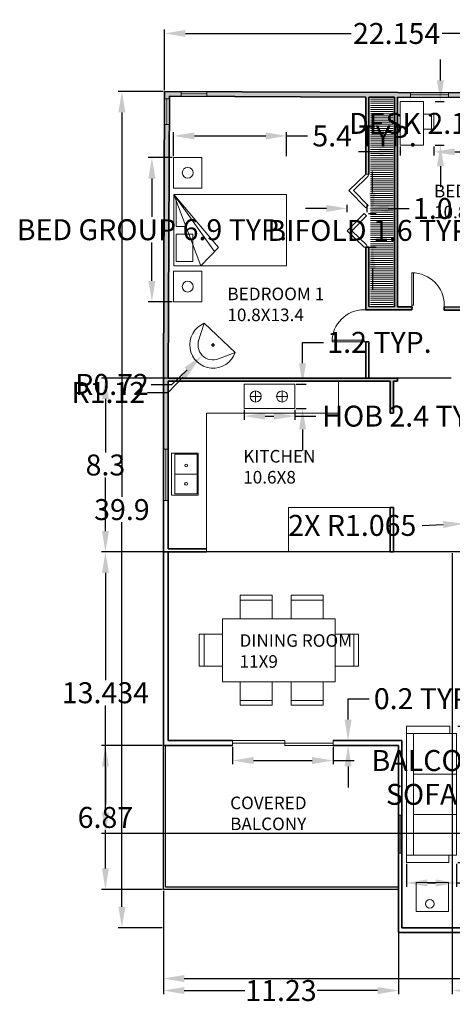
# Model space of a CAD drawing. Units: metres. Extents: x 25.1 to 96.1, y 24.3 to 71.3.
# Tile 1 of 5: x 25.1 to 45.8, y 24.3 to 71.3. Entities that reach past the tile are written whole.
import ezdxf

# ---------------------------------------------------------------- set-up
doc = ezdxf.new("R2010")
doc.units = ezdxf.units.M
doc.header["$MEASUREMENT"] = 0
for name, color, linetype, lineweight in [('A-AREA-IDEN', 1, 'Continuous', 18), ('A-EQPM', 163, 'Continuous', 18), ('A-FLOR-CASE', 8, 'Continuous', 18), ('A-FLOR-FIXT', 163, 'Continuous', 18), ('A-FLOR-RAIL', 7, 'Continuous', 25), ('A-GLAZ', 4, 'Continuous', 18), ('A-WALL', 7, 'Continuous', 35), ('A-WALL-PATT', 252, 'Continuous', 13), ('dimension', 80, 'Continuous', 18), ('door', 17, 'Continuous', 18), ('furniture', 163, 'Continuous', 18)]:
    doc.layers.add(name, color=color, linetype=linetype, lineweight=lineweight)
doc.styles.get("Standard").update_dxf_attribs({"font": 'arial.ttf'})
doc.dimstyles.get("Standard").update_dxf_attribs({"dimtxt": 1, "dimasz": 1, "dimexe": 0.18, "dimexo": 0.0625, "dimgap": 0.09, "dimtad": 0, "dimtih": 1, "dimtoh": 1, "dimdec": 1, "dimzin": 0, "dimdsep": 46, "dimtxsty": 'Standard', "dimcen": 0.09, "dimadec": 0, "dimazin": 0, "dimtfac": 1, "dimtdec": 1, "dimtofl": 0, "dimtmove": 0, "dimatfit": 3, "dimfxl": 1, "dimtolj": 1, "dimtzin": 0, "dimarcsym": 0})

# ---------------------------------------------------------------- blocks, each defined once
blk = doc.blocks.new('*D1')
at = {"layer": 'Defpoints', "color": 0, "transparency": 16777216}
for p in [(30.011, 67.873), (32.047, 67.873), (31.99, 27.968)]:
    blk.add_point(p, dxfattribs=at)
at = {"layer": 'dimension', "color": 0, "lineweight": -2, "transparency": 16777216}
for p, q in [((31.985, 67.873), (29.831, 67.873)), ((30.011, 66.873), (30.011, 48.521)), ((30.011, 28.968), (30.011, 47.319)), ((31.928, 27.968), (29.831, 27.968))]:
    blk.add_line(p, q, dxfattribs=at)
at = {"layer": 'dimension', "color": 0, "transparency": 16777216}
for points in [[(29.844, 66.873), (30.177, 66.873), (30.011, 67.873)], [(29.844, 28.968), (30.177, 28.968), (30.011, 27.968)]]:
    blk.add_solid(points, dxfattribs=at)
at = {"layer": 'dimension', "color": 0, "transparency": 16777216, "insert": (30.011, 47.92), "char_height": 1, "attachment_point": 5}
blk.add_mtext('\\A1;39.9', dxfattribs=at)
blk = doc.blocks.new('s1')
for points in [[(27.599, -10.709), (29.238, -10.709), (29.238, -10.433), (27.599, -10.433)], [(27.863, -10.709), (27.599, -10.709), (27.599, -15.302), (27.863, -15.302)], [(27.863, -10.709), (29.494, -10.709), (29.494, -12.24), (27.863, -12.24)], [(27.863, -12.24), (29.494, -12.24), (29.494, -13.771), (27.863, -13.771)], [(27.863, -13.771), (29.494, -13.771), (29.494, -15.302), (27.863, -15.302)], [(27.599, -15.577), (29.207, -15.577), (29.207, -15.302), (27.599, -15.302)]]:
    blk.add_lwpolyline(points, close=True)
blk = doc.blocks.new('ss')
blk.add_lwpolyline([(27.948, -17.463), (29.489, -17.463), (29.489, -18.849), (27.948, -18.849)], close=True)
blk.add_circle((28.593, -18.475), 0.206)
blk = doc.blocks.new('sink')
for points in [[(16.263, 3.026), (17.543, 3.026), (17.543, 1.019), (16.263, 1.019)], [(17.495, 2.968), (16.431, 2.968), (16.431, 2.028), (17.495, 2.028)], [(17.495, 2.028), (16.431, 2.028), (16.431, 1.081), (17.495, 1.081)]]:
    blk.add_lwpolyline(points, close=True)
for centre in [(16.963, 2.431), (16.961, 1.556)]:
    blk.add_circle(centre, 0.0675)
blk = doc.blocks.new('gas')
for p, q in [((20.016, 5.727), (20.544, 5.727)), ((20.28, 5.991), (20.28, 5.463)), ((21.282, 5.727), (21.81, 5.727)), ((21.546, 5.991), (21.546, 5.463))]:
    blk.add_line(p, q)
blk.add_lwpolyline([(19.729, 6.31), (22.157, 6.31), (22.157, 5.155), (19.729, 5.155)], close=True)
for centre in [(20.28, 5.727), (21.546, 5.727)]:
    blk.add_circle(centre, 0.264)
blk = doc.blocks.new('f')
at = {"layer": 'furniture'}
for p, q in [((25.769, 19.917), (26.843, 19.917)), ((25.769, 19.817), (26.843, 19.817)), ((25.769, 19.717), (26.843, 19.717)), ((25.769, 19.617), (26.843, 19.617)), ((25.769, 19.517), (26.843, 19.517)), ((25.769, 19.417), (26.843, 19.417)), ((25.769, 19.317), (26.843, 19.317)), ((25.769, 19.217), (26.843, 19.217)), ((25.769, 19.117), (26.843, 19.117)), ((25.769, 19.017), (26.843, 19.017)), ((25.769, 18.917), (26.843, 18.917)), ((25.769, 18.817), (26.843, 18.817)), ((25.769, 18.717), (26.843, 18.717)), ((25.769, 18.617), (26.843, 18.617)), ((25.769, 18.517), (26.843, 18.517)), ((25.769, 18.417), (26.843, 18.417)), ((25.769, 18.317), (26.843, 18.317)), ((25.769, 18.217), (26.843, 18.217)), ((25.769, 18.117), (26.843, 18.117)), ((25.769, 18.017), (26.843, 18.017)), ((25.769, 17.917), (26.843, 17.917)), ((25.769, 17.817), (26.843, 17.817)), ((25.769, 17.717), (26.843, 17.717)), ((25.769, 17.617), (26.843, 17.617)), ((25.769, 17.517), (26.843, 17.517)), ((25.769, 17.417), (26.843, 17.417)), ((25.769, 17.317), (26.843, 17.317)), ((25.769, 17.217), (26.843, 17.217)), ((25.769, 17.117), (26.843, 17.117)), ((25.769, 17.017), (26.843, 17.017)), ((25.769, 16.917), (26.843, 16.917)), ((25.769, 16.817), (26.843, 16.817)), ((25.769, 16.717), (26.843, 16.717)), ((25.769, 16.617), (26.843, 16.617)), ((25.769, 16.517), (26.843, 16.517)), ((25.769, 16.417), (26.843, 16.417)), ((25.769, 16.317), (26.843, 16.317)), ((25.769, 16.217), (26.843, 16.217)), ((25.769, 16.117), (26.843, 16.117)), ((25.769, 16.017), (26.843, 16.017)), ((25.769, 15.917), (26.843, 15.917)), ((25.769, 15.817), (26.843, 15.817)), ((25.769, 15.717), (26.843, 15.717)), ((25.769, 15.617), (26.843, 15.617)), ((25.769, 15.517), (26.843, 15.517)), ((25.769, 15.417), (26.843, 15.417)), ((25.769, 15.317), (26.843, 15.317)), ((25.769, 15.217), (26.843, 15.217)), ((25.769, 15.117), (26.843, 15.117)), ((25.769, 15.017), (26.843, 15.017)), ((25.769, 14.917), (26.843, 14.917)), ((25.769, 14.817), (26.843, 14.817)), ((25.769, 14.717), (26.843, 14.717)), ((25.769, 14.617), (26.843, 14.617)), ((25.769, 14.517), (26.843, 14.517)), ((25.769, 14.417), (26.843, 14.417)), ((25.769, 14.317), (26.843, 14.317)), ((25.769, 14.217), (26.843, 14.217)), ((25.769, 14.117), (26.843, 14.117)), ((25.769, 14.017), (26.843, 14.017)), ((25.769, 13.917), (26.843, 13.917)), ((25.769, 13.817), (26.843, 13.817)), ((25.769, 13.717), (26.843, 13.717)), ((25.769, 13.617), (26.843, 13.617)), ((25.769, 13.517), (26.843, 13.517)), ((25.769, 13.417), (26.843, 13.417)), ((25.769, 13.317), (26.843, 13.317)), ((25.769, 13.217), (26.843, 13.217)), ((25.769, 13.117), (26.843, 13.117)), ((25.769, 13.017), (26.843, 13.017)), ((25.769, 12.917), (26.843, 12.917)), ((25.769, 12.817), (26.843, 12.817)), ((25.769, 12.717), (26.843, 12.717)), ((25.769, 12.617), (26.843, 12.617)), ((25.769, 12.517), (26.843, 12.517)), ((25.769, 12.417), (26.843, 12.417)), ((25.769, 12.317), (26.843, 12.317)), ((25.769, 12.217), (26.843, 12.217)), ((25.769, 12.117), (26.843, 12.117)), ((25.769, 12.017), (26.843, 12.017)), ((25.769, 11.917), (26.843, 11.917)), ((25.769, 11.817), (26.843, 11.817)), ((25.769, 11.717), (26.843, 11.717)), ((25.769, 11.617), (26.843, 11.617)), ((25.769, 11.517), (26.843, 11.517)), ((25.769, 11.417), (26.843, 11.417)), ((25.769, 11.317), (26.843, 11.317)), ((25.769, 11.217), (26.843, 11.217)), ((25.769, 11.117), (26.843, 11.117)), ((25.769, 11.017), (26.843, 11.017)), ((25.769, 10.917), (26.843, 10.917)), ((25.769, 10.817), (26.843, 10.817)), ((25.769, 10.717), (26.843, 10.717)), ((25.769, 10.617), (26.843, 10.617)), ((25.769, 10.517), (26.843, 10.517)), ((25.769, 10.417), (26.843, 10.417)), ((25.769, 10.317), (26.843, 10.317)), ((25.769, 10.217), (26.843, 10.217)), ((25.769, 10.117), (26.843, 10.117))]:
    blk.add_line(p, q, dxfattribs=at)
blk = doc.blocks.new('b')
for p, q in [((16.374, 15.368), (18.513, 12.83)), ((17.666, 11.96), (16.374, 15.368)), ((16.374, 15.368), (18.324, 12.637)), ((18.513, 12.83), (17.666, 11.96))]:
    blk.add_line(p, q)
for points in [[(16.362, 17.126), (17.718, 17.126), (17.718, 15.669), (16.362, 15.669)], [(16.374, 15.368), (21.762, 15.368), (21.762, 11.96), (16.374, 11.96)], [(16.486, 12.161), (17.289, 12.161), (17.289, 13.464), (16.486, 13.464)], [(16.362, 11.698), (17.718, 11.698), (17.718, 10.242), (16.362, 10.242)]]:
    blk.add_lwpolyline(points, close=True)
blk.add_lwpolyline([(16.564, 15.144), (16.486, 15.144), (16.486, 13.84), (16.953, 13.84)])
for centre in [(17.04, 16.398), (17.04, 10.97)]:
    blk.add_circle(centre, 0.259)
blk = doc.blocks.new('cc')
for p, q in [((17.83, 9.22), (17.545, 8.337)), ((17.83, 9.22), (19.307, 7.829)), ((19.307, 7.829), (18.516, 7.517))]:
    blk.add_line(p, q)
for radius, start, end in [(1.115, 112.1788, 341.2424), (0.721, 156.2062, 291.5475)]:
    blk.add_arc((18.251, 8.188), radius, start, end)
blk = doc.blocks.new('d')
for p, q in [((25.537, 16.335), (24.732, 15.559)), ((25.644, 16.224), (24.951, 15.555)), ((25.537, 16.335), (25.687, 16.335)), ((25.644, 16.224), (25.687, 16.335)), ((24.732, 15.559), (25.537, 14.725)), ((24.951, 15.555), (25.648, 14.833)), ((25.648, 14.833), (25.537, 14.725))]:
    blk.add_line(p, q)
blk = doc.blocks.new('tt')
for points in [[(27.188, 19.803), (28.295, 19.803), (28.295, 17.712), (27.188, 17.712)], [(28.295, 19.193), (28.681, 19.193), (28.681, 18.478), (28.295, 18.478)], [(28.681, 19.193), (28.789, 19.193), (28.789, 18.478), (28.681, 18.478)]]:
    blk.add_lwpolyline(points, close=True)
blk = doc.blocks.new('*U22')
for p, q in [((0, 0), (0, -6)), ((40, 0), (40, -6))]:
    blk.add_line(p, q)
blk.add_lwpolyline([(0, 0), (0, 40), (1.75, 40), (1.75, 0)], close=True)
blk.add_arc((0, 0), 40, 0, 90)
blk = doc.blocks.new('tttt')
for points in [[(21.475, -3.758), (19.715, -3.758), (19.715, -3.49), (21.475, -3.49)], [(19.715, -4.78), (21.475, -4.78), (21.475, -3.758), (19.715, -3.758)], [(24.267, -3.758), (22.507, -3.758), (22.507, -3.49), (24.267, -3.49)], [(22.507, -4.78), (24.267, -4.78), (24.267, -3.758), (22.507, -3.758)], [(18.746, -4.78), (24.929, -4.78), (24.929, -8.239), (18.746, -8.239)], [(17.724, -5.63), (17.724, -7.389), (17.456, -7.389), (17.456, -5.63)], [(18.746, -7.389), (18.746, -5.63), (17.724, -5.63), (17.724, -7.389)], [(24.929, -7.389), (24.929, -5.63), (25.951, -5.63), (25.951, -7.389)], [(25.951, -5.63), (25.951, -7.389), (26.219, -7.389), (26.219, -5.63)], [(19.715, -8.239), (21.475, -8.239), (21.475, -9.262), (19.715, -9.262)], [(22.507, -8.239), (24.267, -8.239), (24.267, -9.262), (22.507, -9.262)], [(21.475, -9.262), (19.715, -9.262), (19.715, -9.529), (21.475, -9.529)], [(24.267, -9.262), (22.507, -9.262), (22.507, -9.529), (24.267, -9.529)]]:
    blk.add_lwpolyline(points, close=True)
blk = doc.blocks.new('*D24')
at = {"layer": 'Defpoints', "color": 0, "transparency": 16777216}
for p in [(31.99, 29.798), (83.411, 29.798), (83.411, 25.547)]:
    blk.add_point(p, dxfattribs=at)
at = {"layer": 'dimension', "color": 0, "lineweight": -2, "transparency": 16777216}
for p, q in [((31.99, 29.735), (31.99, 25.367)), ((83.411, 29.735), (83.411, 25.367)), ((32.99, 25.547), (56.314, 25.547)), ((82.411, 25.547), (59.087, 25.547))]:
    blk.add_line(p, q, dxfattribs=at)
at = {"layer": 'dimension', "color": 0, "transparency": 16777216}
for points in [[(32.99, 25.713), (32.99, 25.38), (31.99, 25.547)], [(82.411, 25.713), (82.411, 25.38), (83.411, 25.547)]]:
    blk.add_solid(points, dxfattribs=at)
at = {"layer": 'dimension', "color": 0, "transparency": 16777216, "insert": (57.7, 25.547), "char_height": 1, "attachment_point": 5}
blk.add_mtext('\\A1;51.4', dxfattribs=at)
blk = doc.blocks.new('DOOR-BALCONY-SLIDING')
for p, q in [((0, 0.23), (2.501, 0.23)), ((2.501, 0.23), (2.501, 0)), ((2.501, 0), (4.797, 0))]:
    blk.add_line(p, q)
blk.add_lwpolyline([(4.797, 0.115), (4.797, 0.115), (0, 0.115), (0, 0.115)])
blk = doc.blocks.new('*D32')
at = {"layer": 'Defpoints', "color": 0, "transparency": 16777216}
for p in [(41.726, 62.046), (41.726, 60.436), (41.967, 60.436)]:
    blk.add_point(p, dxfattribs=at)
at = {"layer": 'dimension', "color": 0, "lineweight": -2, "transparency": 16777216}
for p, q in [((41.967, 63.046), (41.967, 64.046)), ((41.788, 62.046), (42.147, 62.046)), ((41.788, 60.436), (42.147, 60.436)), ((41.967, 59.436), (41.967, 58.436))]:
    blk.add_line(p, q, dxfattribs=at)
at = {"layer": 'dimension', "color": 0, "transparency": 16777216}
for points in [[(41.801, 63.046), (42.134, 63.046), (41.967, 62.046)], [(41.801, 59.436), (42.134, 59.436), (41.967, 60.436)]]:
    blk.add_solid(points, dxfattribs=at)
at = {"layer": 'dimension', "color": 0, "transparency": 16777216, "insert": (41.967, 61.241), "char_height": 1, "attachment_point": 5}
blk.add_mtext('\\A1;BIFOLD 1.6 TYP.', dxfattribs=at)
blk = doc.blocks.new('*D33')
at = {"layer": 'Defpoints', "color": 0, "transparency": 16777216}
for p in [(40.771, 62.046), (41.726, 62.287), (41.726, 62.046)]:
    blk.add_point(p, dxfattribs=at)
at = {"layer": 'dimension', "color": 0, "lineweight": -2, "transparency": 16777216}
for p, q in [((39.771, 62.287), (38.771, 62.287)), ((40.771, 62.108), (40.771, 62.467)), ((41.726, 62.108), (41.726, 62.467)), ((42.726, 62.287), (43.726, 62.287))]:
    blk.add_line(p, q, dxfattribs=at)
at = {"layer": 'dimension', "color": 0, "transparency": 16777216}
for points in [[(39.771, 62.454), (39.771, 62.121), (40.771, 62.287)], [(42.726, 62.454), (42.726, 62.121), (41.726, 62.287)]]:
    blk.add_solid(points, dxfattribs=at)
at = {"layer": 'dimension', "color": 0, "transparency": 16777216, "insert": (46.397, 62.287), "char_height": 1, "attachment_point": 5}
blk.add_mtext('\\A1;1.0 TYP.', dxfattribs=at)
blk = doc.blocks.new('*D40')
at = {"layer": 'Defpoints', "color": 0, "transparency": 16777216}
for p in [(45.988, 37.586), (46.964, 37.586), (45.988, 31.082)]:
    blk.add_point(p, dxfattribs=at)
at = {"layer": 'dimension', "color": 0, "lineweight": -2, "transparency": 16777216}
for p, q in [((46.051, 37.586), (47.144, 37.586)), ((46.964, 36.586), (46.964, 34.941)), ((46.964, 32.082), (46.964, 33.727)), ((46.051, 31.082), (47.144, 31.082))]:
    blk.add_line(p, q, dxfattribs=at)
at = {"layer": 'dimension', "color": 0, "transparency": 16777216}
for points in [[(46.797, 36.586), (47.13, 36.586), (46.964, 37.586)], [(46.797, 32.082), (47.13, 32.082), (46.964, 31.082)]]:
    blk.add_solid(points, dxfattribs=at)
at = {"layer": 'dimension', "color": 0, "transparency": 16777216, "insert": (46.964, 34.334), "char_height": 1, "attachment_point": 5}
blk.add_mtext('\\A1;SOFA 6.5 TYP.', dxfattribs=at)
blk = doc.blocks.new('*D41')
at = {"layer": 'Defpoints', "color": 0, "transparency": 16777216}
for p in [(43.592, 31.082), (45.988, 31.082), (45.988, 30.107)]:
    blk.add_point(p, dxfattribs=at)
at = {"layer": 'dimension', "color": 0, "lineweight": -2, "transparency": 16777216}
for p, q in [((43.592, 31.02), (43.592, 29.927)), ((45.988, 31.02), (45.988, 29.927)), ((44.592, 30.107), (44.988, 30.107)), ((45.988, 30.107), (46.988, 30.107))]:
    blk.add_line(p, q, dxfattribs=at)
at = {"layer": 'dimension', "color": 0, "transparency": 16777216}
for points in [[(44.592, 30.273), (44.592, 29.94), (43.592, 30.107)], [(44.988, 30.273), (44.988, 29.94), (45.988, 30.107)]]:
    blk.add_solid(points, dxfattribs=at)
at = {"layer": 'dimension', "color": 0, "transparency": 16777216, "insert": (49.714, 30.107), "char_height": 1, "attachment_point": 5}
blk.add_mtext('\\A1;2.4 TYP.', dxfattribs=at)
blk = doc.blocks.new('*D44')
at = {"layer": 'Defpoints', "color": 0, "transparency": 16777216}
for p in [(35.843, 52.744), (38.271, 52.744), (38.271, 52.38)]:
    blk.add_point(p, dxfattribs=at)
at = {"layer": 'dimension', "color": 0, "lineweight": -2, "transparency": 16777216}
for p, q in [((35.843, 52.682), (35.843, 52.2)), ((38.271, 52.682), (38.271, 52.2)), ((36.843, 52.38), (37.271, 52.38)), ((38.271, 52.38), (39.271, 52.38))]:
    blk.add_line(p, q, dxfattribs=at)
at = {"layer": 'dimension', "color": 0, "transparency": 16777216}
for points in [[(36.843, 52.547), (36.843, 52.213), (35.843, 52.38)], [(37.271, 52.547), (37.271, 52.213), (38.271, 52.38)]]:
    blk.add_solid(points, dxfattribs=at)
at = {"layer": 'dimension', "color": 0, "transparency": 16777216, "insert": (43.67, 52.38), "char_height": 1, "attachment_point": 5}
blk.add_mtext('\\A1;HOB 2.4 TYP.', dxfattribs=at)
blk = doc.blocks.new('*D45')
at = {"layer": 'Defpoints', "color": 0, "transparency": 16777216}
for p in [(38.271, 53.899), (38.635, 53.899), (38.271, 52.744)]:
    blk.add_point(p, dxfattribs=at)
at = {"layer": 'dimension', "color": 0, "lineweight": -2, "transparency": 16777216}
for p, q in [((38.635, 54.899), (38.635, 55.899)), ((38.635, 55.899), (39.635, 55.899)), ((38.334, 53.899), (38.815, 53.899)), ((38.334, 52.744), (38.815, 52.744)), ((38.635, 51.744), (38.635, 50.744))]:
    blk.add_line(p, q, dxfattribs=at)
at = {"layer": 'dimension', "color": 0, "transparency": 16777216}
for points in [[(38.469, 54.899), (38.802, 54.899), (38.635, 53.899)], [(38.469, 51.744), (38.802, 51.744), (38.635, 52.744)]]:
    blk.add_solid(points, dxfattribs=at)
at = {"layer": 'dimension', "color": 0, "transparency": 16777216, "insert": (42.306, 55.899), "char_height": 1, "attachment_point": 5}
blk.add_mtext('\\A1;1.2 TYP.', dxfattribs=at)
blk = doc.blocks.new('*D46')
at = {"layer": 'Defpoints', "color": 0, "transparency": 16777216}
for p in [(31.444, 64.716), (32.477, 64.716), (32.477, 57.831)]:
    blk.add_point(p, dxfattribs=at)
at = {"layer": 'dimension', "color": 0, "lineweight": -2, "transparency": 16777216}
for p, q in [((32.414, 64.716), (31.264, 64.716)), ((31.444, 63.716), (31.444, 61.881)), ((31.444, 58.831), (31.444, 60.666)), ((32.414, 57.831), (31.264, 57.831))]:
    blk.add_line(p, q, dxfattribs=at)
at = {"layer": 'dimension', "color": 0, "transparency": 16777216}
for points in [[(31.277, 63.716), (31.611, 63.716), (31.444, 64.716)], [(31.277, 58.831), (31.611, 58.831), (31.444, 57.831)]]:
    blk.add_solid(points, dxfattribs=at)
at = {"layer": 'dimension', "color": 0, "transparency": 16777216, "insert": (31.444, 61.274), "char_height": 1, "attachment_point": 5}
blk.add_mtext('\\A1;BED GROUP 6.9 TYP.', dxfattribs=at)
blk = doc.blocks.new('*D47')
at = {"layer": 'Defpoints', "color": 0, "transparency": 16777216}
for p in [(37.876, 65.748), (32.477, 64.716), (37.876, 64.716)]:
    blk.add_point(p, dxfattribs=at)
at = {"layer": 'dimension', "color": 0, "lineweight": -2, "transparency": 16777216}
for p, q in [((32.477, 64.778), (32.477, 65.928)), ((37.876, 64.778), (37.876, 65.928)), ((33.477, 65.748), (36.876, 65.748)), ((37.876, 65.748), (38.876, 65.748))]:
    blk.add_line(p, q, dxfattribs=at)
at = {"layer": 'dimension', "color": 0, "transparency": 16777216}
for points in [[(33.477, 65.915), (33.477, 65.582), (32.477, 65.748)], [(36.876, 65.915), (36.876, 65.582), (37.876, 65.748)]]:
    blk.add_solid(points, dxfattribs=at)
at = {"layer": 'dimension', "color": 0, "transparency": 16777216, "insert": (41.594, 65.748), "char_height": 1, "attachment_point": 5}
blk.add_mtext('\\A1;5.4 TYP.', dxfattribs=at)
blk = doc.blocks.new('*D52')
at = {"layer": 'Defpoints', "color": 0, "transparency": 16777216}
for p in [(44.903, 67.393), (45.216, 67.393), (44.903, 65.302)]:
    blk.add_point(p, dxfattribs=at)
at = {"layer": 'dimension', "color": 0, "lineweight": -2, "transparency": 16777216}
for p, q in [((45.216, 68.393), (45.216, 69.393)), ((44.965, 67.393), (45.396, 67.393)), ((44.965, 65.302), (45.396, 65.302)), ((45.216, 64.302), (45.216, 63.302))]:
    blk.add_line(p, q, dxfattribs=at)
at = {"layer": 'dimension', "color": 0, "transparency": 16777216}
for points in [[(45.05, 68.393), (45.383, 68.393), (45.216, 67.393)], [(45.05, 64.302), (45.383, 64.302), (45.216, 65.302)]]:
    blk.add_solid(points, dxfattribs=at)
at = {"layer": 'dimension', "color": 0, "transparency": 16777216, "insert": (45.216, 66.348), "char_height": 1, "attachment_point": 5}
blk.add_mtext('\\A1;DESK 2.1 TYP.', dxfattribs=at)
blk = doc.blocks.new('*D53')
at = {"layer": 'Defpoints', "color": 0, "transparency": 16777216}
for p in [(43.302, 65.302), (44.903, 65.302), (44.903, 64.989)]:
    blk.add_point(p, dxfattribs=at)
at = {"layer": 'dimension', "color": 0, "lineweight": -2, "transparency": 16777216}
for p, q in [((42.302, 64.989), (41.302, 64.989)), ((43.302, 65.24), (43.302, 64.809)), ((44.903, 65.24), (44.903, 64.809)), ((45.903, 64.989), (46.903, 64.989))]:
    blk.add_line(p, q, dxfattribs=at)
at = {"layer": 'dimension', "color": 0, "transparency": 16777216}
for points in [[(42.302, 65.155), (42.302, 64.822), (43.302, 64.989)], [(45.903, 65.155), (45.903, 64.822), (44.903, 64.989)]]:
    blk.add_solid(points, dxfattribs=at)
at = {"layer": 'dimension', "color": 0, "transparency": 16777216, "insert": (49.574, 64.989), "char_height": 1, "attachment_point": 5}
blk.add_mtext('\\A1;1.6 TYP.', dxfattribs=at)
blk = doc.blocks.new('*D76')
at = {"layer": 'Defpoints', "color": 0, "transparency": 16777216}
for p in [(35.294, 36.668), (40.091, 36.668), (40.091, 35.948)]:
    blk.add_point(p, dxfattribs=at)
at = {"layer": 'dimension', "color": 0, "lineweight": -2, "transparency": 16777216}
for p, q in [((35.294, 36.605), (35.294, 35.768)), ((40.091, 36.605), (40.091, 35.768)), ((36.294, 35.948), (39.091, 35.948)), ((40.091, 35.948), (41.091, 35.948))]:
    blk.add_line(p, q, dxfattribs=at)
at = {"layer": 'dimension', "color": 0, "transparency": 16777216}
for points in [[(36.294, 36.115), (36.294, 35.781), (35.294, 35.948)], [(39.091, 36.115), (39.091, 35.781), (40.091, 35.948)]]:
    blk.add_solid(points, dxfattribs=at)
at = {"layer": 'dimension', "color": 0, "transparency": 16777216, "insert": (50.036, 35.948), "char_height": 1, "attachment_point": 5}
blk.add_mtext('\\A1;BALCONY SLIDER 4.8 TYP.', dxfattribs=at)
blk = doc.blocks.new('*D77')
at = {"layer": 'Defpoints', "color": 0, "transparency": 16777216}
for p in [(40.091, 36.898), (40.091, 36.668), (40.81, 36.898)]:
    blk.add_point(p, dxfattribs=at)
at = {"layer": 'dimension', "color": 0, "lineweight": -2, "transparency": 16777216}
for p, q in [((40.81, 37.898), (40.81, 38.898)), ((40.81, 38.898), (41.81, 38.898)), ((40.153, 36.898), (40.99, 36.898)), ((40.153, 36.668), (40.99, 36.668)), ((40.81, 35.668), (40.81, 34.668))]:
    blk.add_line(p, q, dxfattribs=at)
at = {"layer": 'dimension', "color": 0, "transparency": 16777216}
for points in [[(40.643, 37.898), (40.977, 37.898), (40.81, 36.898)], [(40.643, 35.668), (40.977, 35.668), (40.81, 36.668)]]:
    blk.add_solid(points, dxfattribs=at)
at = {"layer": 'dimension', "color": 0, "transparency": 16777216, "insert": (44.528, 38.898), "char_height": 1, "attachment_point": 5}
blk.add_mtext('\\A1;0.2 TYP.', dxfattribs=at)
blk = doc.blocks.new('*D78')
at = {"layer": 'Defpoints', "color": 0, "transparency": 16777216}
for p in [(45.784, 45.898), (51.084, 45.898), (51.084, 24.973)]:
    blk.add_point(p, dxfattribs=at)
at = {"layer": 'dimension', "color": 0, "lineweight": -2, "transparency": 16777216}
for p, q in [((45.784, 45.835), (45.784, 24.793)), ((51.084, 45.835), (51.084, 24.793)), ((46.784, 24.973), (47.434, 24.973)), ((50.084, 24.973), (49.434, 24.973))]:
    blk.add_line(p, q, dxfattribs=at)
at = {"layer": 'dimension', "color": 0, "transparency": 16777216}
for points in [[(46.784, 25.139), (46.784, 24.806), (45.784, 24.973)], [(50.084, 25.139), (50.084, 24.806), (51.084, 24.973)]]:
    blk.add_solid(points, dxfattribs=at)
at = {"layer": 'dimension', "color": 0, "transparency": 16777216, "insert": (48.434, 24.973), "char_height": 1, "attachment_point": 5}
blk.add_mtext('\\A1;5.3', dxfattribs=at)
blk = doc.blocks.new('*D80')
at = {"layer": 'Defpoints', "color": 0, "transparency": 16777216}
for p in [(29.225, 54.198), (45.784, 54.198), (45.784, 45.898)]:
    blk.add_point(p, dxfattribs=at)
at = {"layer": 'dimension', "color": 0, "lineweight": -2, "transparency": 16777216}
for p, q in [((45.722, 54.198), (29.045, 54.198)), ((29.225, 53.198), (29.225, 50.648)), ((29.225, 46.898), (29.225, 49.447)), ((45.722, 45.898), (29.045, 45.898))]:
    blk.add_line(p, q, dxfattribs=at)
at = {"layer": 'dimension', "color": 0, "transparency": 16777216}
for points in [[(29.059, 53.198), (29.392, 53.198), (29.225, 54.198)], [(29.059, 46.898), (29.392, 46.898), (29.225, 45.898)]]:
    blk.add_solid(points, dxfattribs=at)
at = {"layer": 'dimension', "color": 0, "transparency": 16777216, "insert": (29.225, 50.048), "char_height": 1, "attachment_point": 5}
blk.add_mtext('\\A1;8.3', dxfattribs=at)
blk = doc.blocks.new('*D81')
at = {"layer": 'Defpoints', "color": 0, "transparency": 16777216}
for p in [(54.201, 70.638), (32.047, 67.873), (54.201, 67.782)]:
    blk.add_point(p, dxfattribs=at)
at = {"layer": 'dimension', "color": 0, "lineweight": -2, "transparency": 16777216}
for p, q in [((32.047, 67.935), (32.047, 70.818)), ((33.047, 70.638), (40.952, 70.638)), ((53.201, 70.638), (45.296, 70.638)), ((54.201, 67.844), (54.201, 70.818))]:
    blk.add_line(p, q, dxfattribs=at)
at = {"layer": 'dimension', "color": 0, "transparency": 16777216}
for points in [[(33.047, 70.804), (33.047, 70.471), (32.047, 70.638)], [(53.201, 70.804), (53.201, 70.471), (54.201, 70.638)]]:
    blk.add_solid(points, dxfattribs=at)
at = {"layer": 'dimension', "color": 0, "transparency": 16777216, "insert": (43.124, 70.638), "char_height": 1, "attachment_point": 5}
blk.add_mtext('\\A1;22.154', dxfattribs=at)
blk = doc.blocks.new('*D82')
at = {"layer": 'Defpoints', "color": 0, "transparency": 16777216}
for p in [(31.99, 29.798), (43.22, 29.798), (43.22, 24.973)]:
    blk.add_point(p, dxfattribs=at)
at = {"layer": 'dimension', "color": 0, "lineweight": -2, "transparency": 16777216}
for p, q in [((31.99, 29.735), (31.99, 24.793)), ((43.22, 29.735), (43.22, 24.793)), ((32.99, 24.973), (35.875, 24.973)), ((42.22, 24.973), (39.335, 24.973))]:
    blk.add_line(p, q, dxfattribs=at)
at = {"layer": 'dimension', "color": 0, "transparency": 16777216}
for points in [[(32.99, 25.139), (32.99, 24.806), (31.99, 24.973)], [(42.22, 25.139), (42.22, 24.806), (43.22, 24.973)]]:
    blk.add_solid(points, dxfattribs=at)
at = {"layer": 'dimension', "color": 0, "transparency": 16777216, "insert": (37.605, 24.973), "char_height": 1, "attachment_point": 5}
blk.add_mtext('\\A1;11.23', dxfattribs=at)
blk = doc.blocks.new('*D83')
at = {"layer": 'Defpoints', "color": 0, "transparency": 16777216}
for p in [(29.225, 36.668), (31.99, 36.668), (31.99, 29.798)]:
    blk.add_point(p, dxfattribs=at)
at = {"layer": 'dimension', "color": 0, "lineweight": -2, "transparency": 16777216}
for p, q in [((31.928, 36.668), (29.045, 36.668)), ((29.225, 35.668), (29.225, 33.833)), ((29.225, 30.798), (29.225, 32.632)), ((31.928, 29.798), (29.045, 29.798))]:
    blk.add_line(p, q, dxfattribs=at)
at = {"layer": 'dimension', "color": 0, "transparency": 16777216}
for points in [[(29.059, 35.668), (29.392, 35.668), (29.225, 36.668)], [(29.059, 30.798), (29.392, 30.798), (29.225, 29.798)]]:
    blk.add_solid(points, dxfattribs=at)
at = {"layer": 'dimension', "color": 0, "transparency": 16777216, "insert": (29.225, 33.233), "char_height": 1, "attachment_point": 5}
blk.add_mtext('\\A1;6.87', dxfattribs=at)
blk = doc.blocks.new('*D84')
at = {"layer": 'Defpoints', "color": 0, "transparency": 16777216}
for p in [(29.225, 45.898), (61.201, 45.898), (61.201, 32.464)]:
    blk.add_point(p, dxfattribs=at)
at = {"layer": 'dimension', "color": 0, "lineweight": -2, "transparency": 16777216}
for p, q in [((61.138, 45.898), (29.045, 45.898)), ((29.225, 44.898), (29.225, 39.781)), ((29.225, 33.464), (29.225, 38.58)), ((61.138, 32.464), (29.045, 32.464))]:
    blk.add_line(p, q, dxfattribs=at)
at = {"layer": 'dimension', "color": 0, "transparency": 16777216}
for points in [[(29.059, 44.898), (29.392, 44.898), (29.225, 45.898)], [(29.059, 33.464), (29.392, 33.464), (29.225, 32.464)]]:
    blk.add_solid(points, dxfattribs=at)
at = {"layer": 'dimension', "color": 0, "transparency": 16777216, "insert": (29.225, 39.181), "char_height": 1, "attachment_point": 5}
blk.add_mtext('\\A1;13.434', dxfattribs=at)
blk = doc.blocks.new('*D88')
at = {"layer": 'Defpoints', "color": 0, "transparency": 16777216}
for p in [(46.349, 47.247), (47.413, 47.29)]:
    blk.add_point(p, dxfattribs=at)
at = {"layer": 'dimension', "color": 0, "lineweight": -2, "transparency": 16777216}
for p, q in [((44.351, 47.166), (45.35, 47.207)), ((47.323, 47.29), (47.503, 47.29)), ((47.413, 47.2), (47.413, 47.38))]:
    blk.add_line(p, q, dxfattribs=at)
at = {"layer": 'dimension', "color": 0, "transparency": 16777216}
blk.add_solid([(45.344, 47.373), (45.357, 47.04), (46.349, 47.247)], dxfattribs=at)
at = {"layer": 'dimension', "color": 0, "transparency": 16777216, "insert": (41.009, 47.166), "char_height": 1, "attachment_point": 5}
blk.add_mtext('\\A1;2X R1.065', dxfattribs=at)
blk = doc.blocks.new('*D89')
at = {"layer": 'Defpoints', "color": 0, "transparency": 16777216}
for p in [(34.365, 55.778), (33.6, 54.966)]:
    blk.add_point(p, dxfattribs=at)
at = {"layer": 'dimension', "color": 0, "lineweight": -2, "transparency": 16777216}
for p, q in [((34.275, 55.778), (34.455, 55.778)), ((34.365, 55.688), (34.365, 55.868)), ((32.228, 53.51), (32.914, 54.238)), ((31.228, 53.51), (32.228, 53.51))]:
    blk.add_line(p, q, dxfattribs=at)
at = {"layer": 'dimension', "color": 0, "transparency": 16777216}
blk.add_solid([(32.793, 54.352), (33.036, 54.124), (33.6, 54.966)], dxfattribs=at)
at = {"layer": 'dimension', "color": 0, "transparency": 16777216, "insert": (29.366, 53.51), "char_height": 1, "attachment_point": 5}
blk.add_mtext('\\A1;R1.12', dxfattribs=at)
blk = doc.blocks.new('*D90')
at = {"layer": 'Defpoints', "color": 0, "transparency": 16777216}
for p in [(34.365, 55.778), (33.845, 55.278)]:
    blk.add_point(p, dxfattribs=at)
at = {"layer": 'dimension', "color": 0, "lineweight": -2, "transparency": 16777216}
for p, q in [((34.275, 55.778), (34.455, 55.778)), ((34.365, 55.688), (34.365, 55.868)), ((32.403, 53.892), (33.124, 54.585)), ((31.403, 53.892), (32.403, 53.892))]:
    blk.add_line(p, q, dxfattribs=at)
at = {"layer": 'dimension', "color": 0, "transparency": 16777216}
blk.add_solid([(33.008, 54.705), (33.239, 54.465), (33.845, 55.278)], dxfattribs=at)
at = {"layer": 'dimension', "color": 0, "transparency": 16777216, "insert": (29.541, 53.892), "char_height": 1, "attachment_point": 5}
blk.add_mtext('\\A1;R0.72', dxfattribs=at)

msp = doc.modelspace()

# ---------------------------------------------------------------- hatches: boundary and pattern name
at = {"layer": 'A-WALL-PATT'}
h = msp.add_hatch(color=256, dxfattribs=at)
h.dxf.hatch_style = 1
h.paths.add_polyline_path([(32.2705, 66.2918), (32.0405, 66.2928), (31.9902, 54.0475), (31.9902, 50.7969), (32.2202, 50.7969), (32.2202, 54.0475), (42.8202, 54.0475), (42.8202, 52.5275), (42.9702, 52.5275), (42.9702, 54.0475), (43.1708, 54.0475), (43.1708, 54.1975), (32.2208, 54.1975)])
h.paths.add_polyline_path([(32.8404, 67.8694), (32.047, 67.8727), (32.0456, 67.5128), (32.2756, 67.5118), (32.2761, 67.6417), (32.8395, 67.6394)])
h.paths.add_polyline_path([(43.7857, 67.8244), (34.0604, 67.8644), (34.0595, 67.6344), (41.6508, 67.6032), (41.6508, 63.9251), (41.8008, 63.9251), (41.8008, 67.6026), (43.0208, 67.5975), (43.0208, 57.5975), (41.8008, 57.6025), (41.8008, 60.436), (41.6508, 60.436), (41.6508, 57.4531), (43.8592, 57.444), (43.8592, 57.594), (43.1708, 57.5968), (43.1708, 67.5969), (43.7848, 67.5944)])
h.paths.add_polyline_path([(56.5108, 67.7816), (54.2008, 67.7816), (45.5957, 67.8169), (45.5947, 67.5869), (53.9708, 67.5525), (53.9708, 58.9224), (52.4515, 58.9287), (52.4508, 58.779), (52.4512, 58.7787), (53.9708, 58.7724), (53.9708, 57.5524), (49.0027, 57.5728), (49.0077, 58.7928), (50.2244, 58.7878), (50.2244, 58.9378), (48.8584, 58.9435), (48.8577, 58.7935), (48.8527, 57.5735), (45.4006, 57.5877), (45.4006, 57.4377), (53.9634, 57.4024), (54.2008, 57.4024), (54.2008, 67.5516), (56.5108, 67.5516)])
h.paths.add_polyline_path([(68.3657, 67.7816), (58.8908, 67.7816), (58.8908, 67.5516), (61.2008, 67.5516), (61.2008, 57.4016), (61.4308, 57.4016), (67.4455, 57.4016), (67.4455, 58.9016), (66.0112, 58.9016), (66.0112, 58.7516), (67.2955, 58.7516), (67.2955, 57.5516), (61.4308, 57.5516), (61.4308, 58.7516), (63.7844, 58.7516), (63.7844, 58.9016), (61.4308, 58.9016), (61.4308, 67.5516), (68.3657, 67.5516)])

# ---------------------------------------------------------------- linework, layer by layer
at = {"layer": 'A-FLOR-CASE'}
for p, q in [((40.3575, 52.5275), (40.3575, 54.0475)), ((34.0502, 45.8975), (34.0502, 52.5275)), ((40.3575, 52.5275), (34.0502, 52.5275))]:
    msp.add_line(p, q, dxfattribs=at)
msp.add_lwpolyline([(42.8202, 45.8975), (42.8202, 48.0275), (37.9709, 48.0275), (37.9709, 45.8975), (42.8202, 45.8975)], dxfattribs=at)
at = {"layer": 'A-FLOR-RAIL'}
for p, q in [((31.9902, 29.7975), (31.9902, 36.6675)), ((32.0902, 29.8975), (32.0902, 36.6675)), ((43.2202, 29.7975), (31.9902, 29.7975)), ((43.2202, 29.8975), (32.0902, 29.8975))]:
    msp.add_line(p, q, dxfattribs=at)
at = {"layer": 'A-GLAZ'}
for p, q in [((32.8395, 67.6394), (32.8404, 67.8694)), ((34.0599, 67.7494), (32.8399, 67.7544)), ((34.0595, 67.6344), (34.0604, 67.8644)), ((43.7848, 67.5944), (43.7857, 67.8244)), ((43.7852, 67.7094), (45.5952, 67.7019)), ((45.5947, 67.5869), (45.5957, 67.8169)), ((32.2756, 67.5118), (32.0456, 67.5128)), ((32.1555, 66.2923), (32.1606, 67.5123)), ((32.2705, 66.2918), (32.0405, 66.2928)), ((32.2202, 50.7969), (31.9902, 50.7969)), ((32.1052, 50.7969), (32.1052, 48.3569)), ((32.2202, 48.3569), (31.9902, 48.3569)), ((43.3702, 33.3425), (43.2202, 33.3425)), ((43.2952, 31.5225), (43.2952, 33.3425)), ((43.3702, 31.5225), (43.2202, 31.5225))]:
    msp.add_line(p, q, dxfattribs=at)
at = {"layer": 'A-WALL'}
for p, q in [((31.9902, 54.0475), (32.047, 67.8727)), ((32.047, 67.8727), (54.2008, 67.7816)), ((32.2208, 54.1975), (32.2761, 67.6417)), ((32.2761, 67.6417), (41.6508, 67.6032)), ((41.6508, 67.6032), (41.6508, 63.9251)), ((41.8008, 67.6026), (41.8008, 63.9251)), ((41.8008, 67.6026), (43.0208, 67.5975)), ((43.0208, 67.5975), (43.0208, 57.5975)), ((43.1708, 67.5969), (43.1708, 57.5968)), ((43.1708, 67.5969), (53.9708, 67.5525)), ((41.6508, 60.6092), (41.6508, 60.6092)), ((41.6508, 60.436), (41.8008, 60.436)), ((41.6508, 60.436), (41.6508, 57.4531)), ((41.8008, 60.436), (41.8008, 57.6025)), ((41.6508, 57.4531), (43.8592, 57.444)), ((41.8008, 57.6025), (43.0208, 57.5975)), ((43.1708, 57.5968), (43.8598, 57.594)), ((43.8598, 57.594), (43.8592, 57.444)), ((45.3998, 57.5877), (45.3992, 57.4377)), ((45.3992, 57.4377), (53.9708, 57.4024)), ((45.3998, 57.5877), (48.8527, 57.5735)), ((41.6508, 55.93), (41.6508, 54.1975)), ((41.8008, 55.93), (41.6508, 55.93)), ((41.8008, 55.93), (41.8008, 54.1975)), ((31.9902, 36.6675), (31.9902, 54.0475)), ((32.2202, 46.0475), (32.2202, 54.0475)), ((42.8202, 54.0475), (32.2202, 54.0475)), ((43.1708, 54.1975), (32.2208, 54.1975)), ((42.8202, 52.5275), (42.8202, 54.0475)), ((43.1708, 54.0475), (42.9702, 54.0475)), ((42.9702, 52.5275), (42.9702, 54.0475)), ((43.1708, 54.1975), (43.1708, 54.0475)), ((42.8202, 52.5275), (42.9702, 52.5275)), ((42.8202, 45.8975), (42.8202, 48.0275)), ((42.9702, 48.0275), (42.8202, 48.0275)), ((42.9702, 45.8975), (42.9702, 48.0275)), ((34.0502, 46.0475), (32.2202, 46.0475)), ((34.0502, 45.8975), (31.9902, 45.8975)), ((32.2202, 36.8975), (32.2202, 45.8975)), ((42.9702, 45.8975), (42.8202, 45.8975)), ((35.2938, 36.6675), (31.9902, 36.6675)), ((35.2938, 36.8975), (32.2202, 36.8975)), ((43.3702, 36.8975), (40.0906, 36.8975)), ((43.2202, 36.6675), (40.0906, 36.6675)), ((43.2202, 29.8975), (43.2202, 36.6675)), ((43.3702, 27.9675), (43.3702, 36.8975)), ((43.2202, 27.7375), (43.2202, 29.8975)), ((54.2008, 27.7375), (43.2202, 27.7375)), ((53.9708, 27.9675), (43.3702, 27.9675))]:
    msp.add_line(p, q, dxfattribs=at)
at = {"layer": 'door'}
for p, q in [((35.2938, 36.6675), (35.2938, 36.8975)), ((40.0906, 36.6675), (40.0906, 36.8975))]:
    msp.add_line(p, q, dxfattribs=at)

# ---------------------------------------------------------------- block references
at = {"layer": 'A-EQPM'}
msp.add_blockref('gas', (16.1141, 47.5898), dxfattribs=at)
at = {"layer": 'A-FLOR-CASE'}
msp.add_blockref('f', (16.1141, 47.5898), dxfattribs=at)
msp.add_blockref('f', (16.1141, 47.5898), dxfattribs=at)
at = {"layer": 'A-FLOR-FIXT'}
msp.add_blockref('sink', (16.1141, 47.5898), dxfattribs=at)
at = {"layer": 'door'}
for name, p in [('d', (16.1141, 47.5898)), ('DOOR-BALCONY-SLIDING', (35.294, 36.668))]:
    msp.add_blockref(name, p, dxfattribs=at)
at = {"layer": 'door', "xscale": -1, "rotation": 180}
msp.add_blockref('d', (16.0391, 76.7713), dxfattribs=at)
at = {"layer": 'door', "xscale": 0.0385366420547583, "yscale": 0.0385366420547583, "zscale": 0.0385366420547583}
msp.add_blockref('*U22', (43.8592, 57.6752), dxfattribs=at)
at = {"layer": 'door', "xscale": 0.0381340016713186, "yscale": 0.0381340016713186, "zscale": 0.0381340016713186, "rotation": 90}
msp.add_blockref('*U22', (41.572, 55.93), dxfattribs=at)
at = {"layer": 'furniture'}
for name in ['tt', 'b', 'cc', 'ss']:
    msp.add_blockref(name, (16.1141, 47.5898), dxfattribs=at)
for name, p, xscale, yscale, zscale in [('tttt', (18.5321, 46.8655), 0.8688370319284477, 0.8688370319284477, 0.8688370319284477), ('s1', (8.6961, 50.7774), 1.264373167528455, 1.264373167528455, 1.264373167528455)]:
    msp.add_blockref(name, p, dxfattribs=dict(at, xscale=xscale, yscale=yscale, zscale=zscale))

# ---------------------------------------------------------------- texts
at = {"layer": 'A-AREA-IDEN', "char_height": 0.6, "attachment_point": 1}
for s, width, insert in [('BEDROOM 2\\P10.8X10', 5.007262, (44.9092, 63.415)), ('BEDROOM 1\\P10.8X13.4', 5.007262, (35.0481, 58.511)), ('KITCHEN\\P10.6X8', 5.007262, (35.802, 50.7644)), ('DINING ROOM\\P11X9', 11.597488, (35.628, 41.9738)), ('COVERED\\PBALCONY', 5.007262, (35.1792, 34.2251))]:
    msp.add_mtext_dynamic_manual_height_columns(s, width=width, gutter_width=1, heights=[0], dxfattribs=dict(at, insert=insert))

# ---------------------------------------------------------------- dimensions: what is measured, and where the dimension line sits
at = {"layer": 'dimension'}
for base, p1, p2, override, picture, middle in [((54.2008, 70.6377), (32.047, 67.8727), (54.2008, 67.7816), {"dimdec": 3, "dimlfac": 1, "dimrnd": 0, "dimzin": 0, "dimdsep": 46, "dimlunit": 2}, '*D81', (43.1239, 70.6377)), ((51.0841, 24.9725), (45.7841, 45.8975), (51.0841, 45.8975), {"dimdec": 1, "dimlfac": 1, "dimrnd": 0, "dimzin": 0, "dimdsep": 46, "dimlunit": 2}, '*D78', (48.4341, 24.9725)), ((83.4108, 25.5466), (31.9902, 29.7975), (83.4108, 29.7975), {"dimclrd": 0, "dimclre": 0, "dimclrt": 0}, '*D24', (57.7005, 25.5466)), ((43.2202, 24.9725), (31.9902, 29.7975), (43.2202, 29.7975), {"dimdec": 2, "dimlfac": 1, "dimrnd": 0, "dimzin": 0, "dimdsep": 46, "dimlunit": 2}, '*D82', (37.6052, 24.9725))]:
    dim = msp.add_linear_dim(base=base, p1=p1, p2=p2, dimstyle='Standard', override=override, dxfattribs=at)
    dim.commit()
    dim.dimension.update_dxf_attribs({"geometry": picture, "text_midpoint": middle})
for base, p1, p2, angle, text, picture, middle in [((45.2164, 67.393), (44.9028, 65.3022), (44.9028, 67.393), 90, 'DESK <> TYP.', '*D52', (45.2164, 66.3476)), ((31.4439, 64.7158), (32.4766, 57.8315), (32.4766, 64.7158), 90, 'BED GROUP <> TYP.', '*D46', (31.4439, 61.2736)), ((41.9673, 60.436), (41.7258, 62.0459), (41.7258, 60.436), 270, 'BIFOLD <> TYP.', '*D32', (41.9673, 61.241)), ((38.6354, 53.8994), (38.2712, 52.7443), (38.2712, 53.8994), 90, '<> TYP.', '*D45', (42.3062, 55.8994)), ((40.8101, 36.8975), (40.0906, 36.6675), (40.0906, 36.8975), 90, '<> TYP.', '*D77', (44.528, 38.8975)), ((46.9636, 37.5858), (45.9881, 31.0821), (45.9881, 37.5858), 90, 'SOFA <> TYP.', '*D40', (46.9636, 34.3339))]:
    dim = msp.add_linear_dim(base=base, p1=p1, p2=p2, angle=angle, text=text, dimstyle='Standard', override={"dimdec": 1, "dimlfac": 1, "dimrnd": 0, "dimzin": 0, "dimdsep": 46, "dimlunit": 2}, dxfattribs=at)
    dim.commit()
    dim.dimension.update_dxf_attribs({"geometry": picture, "text_midpoint": middle})
for base, p1, p2, override, picture, middle in [((30.0108, 67.8727), (31.9903, 27.9675), (32.047, 67.8727), {"dimclrd": 0, "dimclre": 0, "dimclrt": 0}, '*D1', (30.0108, 47.9201)), ((29.2252, 54.1975), (45.7841, 45.8975), (45.7841, 54.1975), {"dimdec": 1, "dimlfac": 1, "dimrnd": 0, "dimzin": 0, "dimdsep": 46, "dimlunit": 2}, '*D80', (29.2252, 50.0475)), ((29.2252, 45.8975), (61.2008, 32.4635), (61.2008, 45.8975), {"dimdec": 3, "dimlfac": 1, "dimrnd": 0, "dimzin": 0, "dimdsep": 46, "dimlunit": 2}, '*D84', (29.2252, 39.1805)), ((29.2252, 36.6675), (31.9902, 29.7975), (31.9902, 36.6675), {"dimdec": 2, "dimlfac": 1, "dimrnd": 0, "dimzin": 0, "dimdsep": 46, "dimlunit": 2}, '*D83', (29.2252, 33.2325))]:
    dim = msp.add_linear_dim(base=base, p1=p1, p2=p2, angle=90, dimstyle='Standard', override=override, dxfattribs=at)
    dim.commit()
    dim.dimension.update_dxf_attribs({"geometry": picture, "text_midpoint": middle})
for base, p1, p2, text, picture, middle in [((37.8758, 65.7485), (32.4766, 64.7158), (37.8758, 64.7158), '<> TYP.', '*D47', (41.5937, 65.7485)), ((44.9028, 64.9886), (43.3025, 65.3022), (44.9028, 65.3022), '<> TYP.', '*D53', (49.5736, 64.9886)), ((41.7258, 62.2874), (40.7713, 62.0459), (41.7258, 62.0459), '<> TYP.', '*D33', (46.3966, 62.2874)), ((38.2712, 52.3801), (35.8431, 52.7443), (38.2712, 52.7443), 'HOB <> TYP.', '*D44', (43.6698, 52.3801)), ((40.0906, 35.948), (35.2938, 36.6675), (40.0906, 36.6675), 'BALCONY SLIDER <> TYP.', '*D76', (50.036, 35.948)), ((45.9881, 30.1065), (43.5915, 31.0821), (45.9881, 31.0821), '<> TYP.', '*D41', (49.7145, 30.1065))]:
    dim = msp.add_linear_dim(base=base, p1=p1, p2=p2, text=text, dimstyle='Standard', override={"dimdec": 1, "dimlfac": 1, "dimrnd": 0, "dimzin": 0, "dimdsep": 46, "dimlunit": 2}, dxfattribs=at)
    dim.commit()
    dim.dimension.update_dxf_attribs({"geometry": picture, "text_midpoint": middle})
for mpoint, picture, middle in [((33.6, 54.966), '*D89', (29.3663, 53.5104)), ((33.8447, 55.2777), '*D90', (29.5407, 53.8917))]:
    dim = msp.add_radius_dim(center=(34.3647, 55.7776), mpoint=mpoint, dimstyle='Standard', override={"dimdec": 2, "dimlfac": 1, "dimrnd": 0, "dimzin": 0, "dimdsep": 46, "dimlunit": 2}, dxfattribs=at)
    dim.commit()
    dim.dimension.update_dxf_attribs({"geometry": picture, "text_midpoint": middle})
dim = msp.add_radius_dim(center=(47.4135, 47.2899), mpoint=(46.3494, 47.247), text='2X <>', dimstyle='Standard', override={"dimdec": 3, "dimlfac": 1, "dimrnd": 0, "dimzin": 0, "dimdsep": 46, "dimlunit": 2}, dxfattribs=at)
dim.commit()
dim.dimension.update_dxf_attribs({"geometry": '*D88', "text_midpoint": (41.0086, 47.1664)})

doc.saveas('drawing.dxf')
